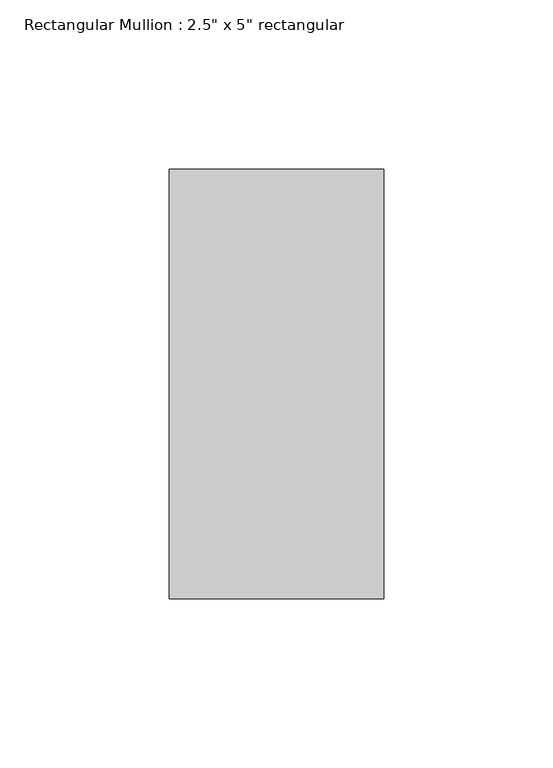
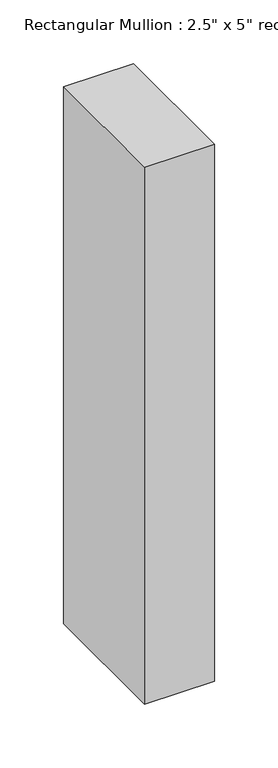
"""IFC4 building model written with IfcOpenShell, lengths in millimetres: member geometry."""

from ifc_helpers import new_model, si_unit, frame, origin, place, context, project, spatial, polyline, outline, extrude, source, transform, mapped, element, save


def member_aaa03826(model_context):
    return source(origin(), model_context, "Body", "SweptSolid", [
        extrude(outline(polyline([(31.75, 63.5), (31.75, -63.5), (-31.75, -63.5), (-31.75, 63.5), (31.75, 63.5)])), frame((0.0, 0.0, -514.35), z_axis=(0.0, 0.0, 1.0), x_axis=(1.0, 0.0, 0.0)), (0.0, 0.0, 1.0), 514.35),
    ])


if __name__ == "__main__":
    model = new_model("IFC4")
    model_context = context("Model", 3, world=origin())
    ifc_project = project(units=[si_unit("LENGTHUNIT", "METRE", prefix="MILLI")], contexts=[model_context])
    site = spatial("IfcSite", under=ifc_project)
    building = spatial("IfcBuilding", under=site)
    placement = place(None, origin())
    member_shape = member_aaa03826(model_context)
    element("IfcMember", 1, ObjectType="Rectangular Mullion : 2.5\" x 5\" rectangular", at=placement, inside=building, context=model_context, shape_type="MappedRepresentation", body=[
        mapped(member_shape, transform((0.0, 0.0, 0.0), x_axis=(1.0, 0.0, 0.0), y_axis=(0.0, 1.0, 0.0), z_axis=(0.0, 0.0, 1.0))),
    ])
    save(model, "model.ifc")

# Revit data of these elements
# Type "Rectangular Mullion : 2.5\" x 5\" rectangular"
#   built-in parameter 1007304 = 0.416667 (stored number, unit not read)
#   built-in parameter 1007301 = 0.104167 (stored number, unit not read)
#   built-in parameter 1007300 = 0.104167 (stored number, unit not read)
# Element 1 (IfcMember, "Rectangular Mullion : 2.5\" x 5\" rectangular")
#   Materials on its faces: "Damp-proofing"
# Materials
#   "Damp-proofing": class "Generic", colour RGB 127 127 127, transparency 0, Description = "Damp-proofing", Cost = 0
